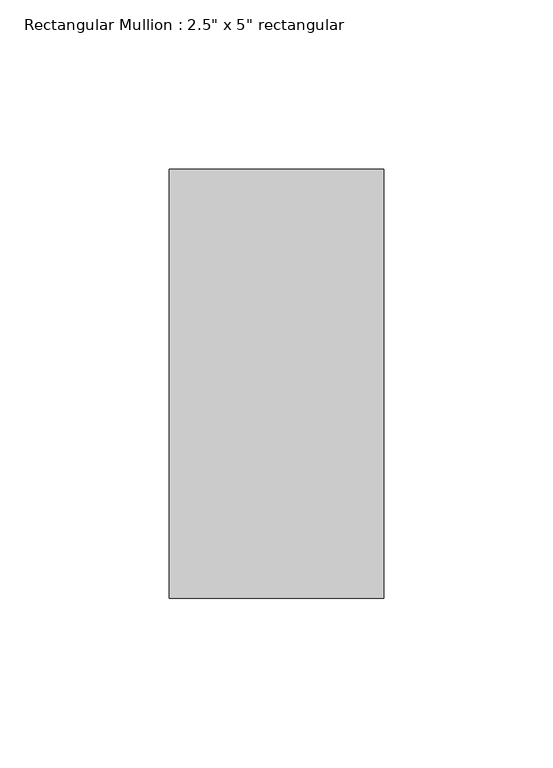
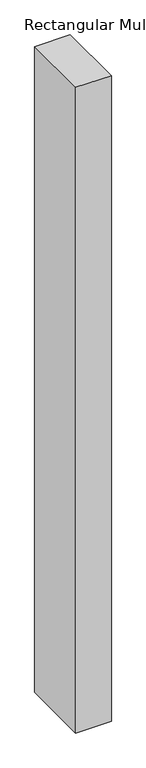
"""IFC4 building model written with IfcOpenShell, lengths in millimetres: member geometry."""

from ifc_helpers import new_model, si_unit, frame, origin, place, context, project, spatial, polyline, outline, extrude, source, transform, mapped, element, save


def member_75074519(model_context):
    return source(origin(), model_context, "Body", "SweptSolid", [
        extrude(outline(polyline([(0.0, 63.5), (0.0, -63.5), (-63.5, -63.5), (-63.5, 63.5), (0.0, 63.5)])), frame((0.0, 0.0, -1219.2), z_axis=(0.0, 0.0, 1.0), x_axis=(1.0, 0.0, 0.0)), (0.0, 0.0, 1.0), 1219.2),
    ])


if __name__ == "__main__":
    model = new_model("IFC4")
    model_context = context("Model", 3, world=origin())
    ifc_project = project(units=[si_unit("LENGTHUNIT", "METRE", prefix="MILLI")], contexts=[model_context])
    site = spatial("IfcSite", under=ifc_project)
    building = spatial("IfcBuilding", under=site)
    placement = place(None, origin())
    member_shape = member_75074519(model_context)
    element("IfcMember", 1, ObjectType="Rectangular Mullion : 2.5\" x 5\" rectangular", at=placement, inside=building, context=model_context, shape_type="MappedRepresentation", body=[
        mapped(member_shape, transform((0.0, 0.0, 0.0), x_axis=(1.0, 0.0, 0.0), y_axis=(0.0, 1.0, 0.0), z_axis=(0.0, 0.0, 1.0))),
    ])
    save(model, "model.ifc")

# Revit data of these elements
# Type "Rectangular Mullion : 2.5\" x 5\" rectangular"
#   built-in parameter 1007304 = 0.416667 (stored number, unit not read)
#   built-in parameter 1007301 = 0.104167 (stored number, unit not read)
#   built-in parameter 1007300 = 0.104167 (stored number, unit not read)
